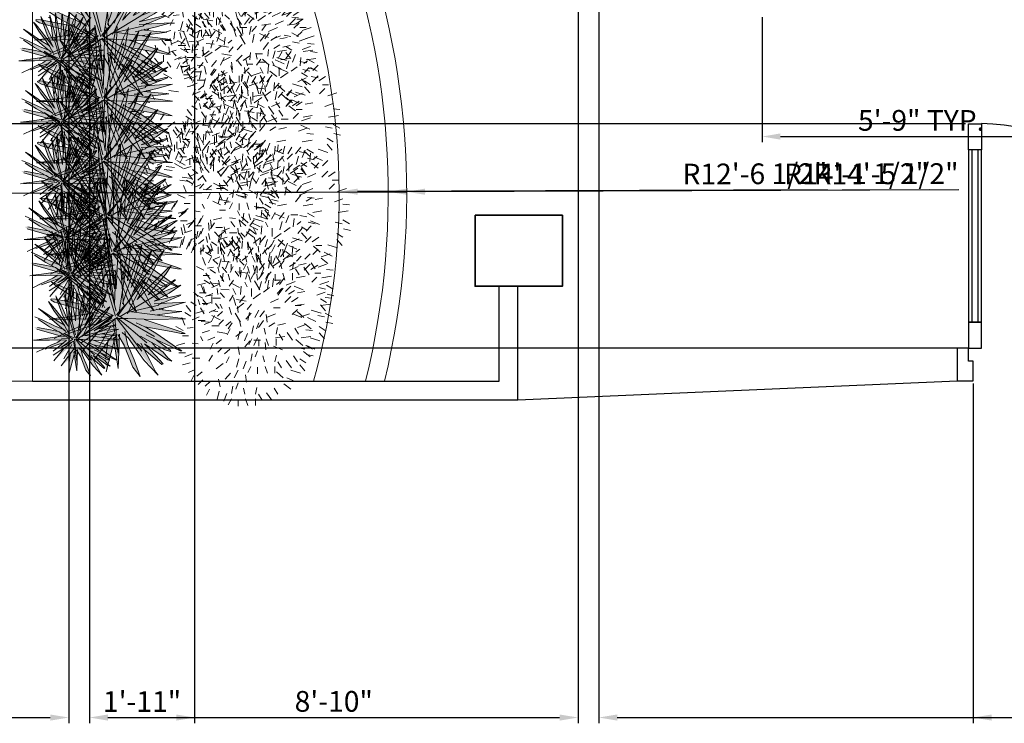
# Model space of a CAD drawing. Units: inches. Extents: x 1239 to 2276906, y 2273 to 321338.
# Tile 6 of 23: x 1541 to 1754, y 2276 to 2428. Entities that reach past the tile are written whole.
import ezdxf

# ---------------------------------------------------------------- set-up
doc = ezdxf.new("R2010")
doc.units = ezdxf.units.IN
for name, color, linetype, lineweight in [('A-ANNO-DIMS', 2, 'Continuous', 18), ('A-COLS', 7, 'Continuous', 35), ('C-PROP', 7, 'Continuous', 25), ('L-PLNT', 94, 'Continuous', 13), ('L-SITE-GATE', 1, 'Continuous', 25)]:
    doc.layers.add(name, color=color, linetype=linetype, lineweight=lineweight)
doc.styles.get("Standard").update_dxf_attribs({"font": 'arial.ttf'})
doc.dimstyles.new('ISO-25', dxfattribs={"dimtxt": 4.5, "dimasz": 4, "dimexe": 1.25, "dimexo": 0.625, "dimtad": 1, "dimdec": 1, "dimlunit": 3, "dimtxsty": 'Standard', "dimcen": 2.5, "dimadec": 0, "dimazin": 0, "dimtfac": 1, "dimtdec": 1, "dimtmove": 0, "dimatfit": 3, "dimfxl": 1, "dimarcsym": 0})

# ---------------------------------------------------------------- blocks, each defined once
blk = doc.blocks.new('A$C545C060E')
h = blk.add_hatch(color=256)
h.set_gradient(color1=(31, 127, 0), color2=(45, 179, 0), one_color=1, tint=0.35, name='INVSPHERICAL')
h.paths.add_polyline_path([(0.529, 2.393), (0.645, 2.304), (1.889, 1.967), (0.489, 1.77), (1.843, 1.787), (1.618, 1.643), (0.635, 1.178), (1.063, 1.326), (1.966, 1.643), (1.461, 1.231), (1.869, 1.417), (2.379, 1.664), (2.177, 1.5), (1.446, 1.03), (1.981, 1.358), (1.481, 0.744), (2.376, 1.553), (1.986, 0.848), (2.48, 1.336), (1.85, 0.496), (2.266, 0.842), (2.223, 0.533), (2.243, 0.142), (2.487, 1.093), (2.615, 0.257), (2.655, 1.214), (3.074, 0.284), (3.303, 0), (2.908, 1.003), (2.846, 1.271), (2.929, 1.199), (3.853, 0.038), (3.428, 0.832), (3.973, 0.376), (4.009, 0.393), (3.432, 1.008), (3.923, 0.676), (4.175, 0.507), (4.274, 0.474), (4.155, 0.583), (4.009, 0.757), (3.765, 0.932), (3.662, 1.051), (4.067, 0.828), (4.243, 0.779), (4.238, 0.801), (3.802, 1.133), (4.534, 0.795), (4.591, 0.795), (4.42, 0.899), (4.103, 1.12), (3.786, 1.34), (3.464, 1.533), (3.968, 1.441), (4.415, 1.362), (4.571, 1.335), (4.695, 1.33), (3.997, 1.572), (3.423, 1.771), (4.695, 1.782), (3.833, 1.912), (4.591, 2.011), (3.836, 2.079), (4.706, 2.305), (3.951, 2.263), (4.55, 2.506), (4.555, 2.528), (4.493, 2.517), (3.734, 2.332), (4.197, 2.577), (4.56, 2.833), (3.786, 2.523), (4.363, 2.959), (4.394, 2.997), (4.363, 2.997), (3.558, 2.528), (3.549, 2.536), (4.087, 3.155), (4.254, 3.422), (4.191, 3.389), (3.209, 2.381), (4.046, 3.912), (3.999, 3.874), (3.09, 2.626), (3.547, 3.58), (3.666, 3.934), (3.35, 3.438), (3.017, 2.752), (3.225, 3.411), (3.345, 4.064), (3.243, 3.868), (3.184, 3.754), (2.919, 3.073), (2.986, 3.83), (2.991, 4.097), (2.96, 4.075), (2.742, 2.981), (2.732, 2.92), (2.659, 4.026), (2.633, 4.092), (2.612, 4.005), (2.56, 2.719), (2.3, 4.135), (2.382, 2.743), (2.025, 4.026), (2.02, 3.934), (1.968, 3.917), (2.046, 3.874), (2.185, 2.776), (1.976, 3.197), (1.829, 3.524), (1.673, 3.773), (1.577, 3.963), (1.613, 3.821), (1.751, 3.44), (1.89, 3.059), (2.192, 2.446), (1.345, 3.551), (1.215, 3.683), (1.481, 3.234), (2.006, 2.515), (1.567, 2.769), (0.983, 3.176), (0.731, 3.334), (1.255, 2.901), (1.969, 2.294), (0.912, 2.769), (0.549, 2.927), (1.687, 2.199), (0.675, 2.399), (0.554, 2.409)])
h = blk.add_hatch(color=256)
h.set_gradient(color1=(31, 127, 0), color2=(55, 219, 0), one_color=1, tint=0.43, name='SPHERICAL')
h.paths.add_polyline_path([(3.023, 2.188), (3.114, 2.362), (3.471, 3.049), (3.33, 2.866), (2.618, 1.891), (2.679, 1.855), (2.94, 2.013)])
h = blk.add_hatch(color=256)
h.set_gradient(color1=(31, 127, 0), color2=(45, 179, 0), one_color=1, tint=0.35, name='INVSPHERICAL')
h.paths.add_polyline_path([(0.025, 1.517), (0.098, 1.461), (0.877, 1.25), (0, 1.126), (0.848, 1.137), (0.707, 1.047), (0.092, 0.756), (0.36, 0.848), (0.925, 1.047), (0.609, 0.789), (0.865, 0.905), (1.184, 1.06), (1.058, 0.958), (0.6, 0.663), (0.935, 0.868), (0.622, 0.484), (1.182, 0.99), (0.938, 0.549), (1.247, 0.855), (0.853, 0.328), (1.113, 0.545), (1.086, 0.352), (1.099, 0.106), (1.252, 0.703), (1.332, 0.179), (1.357, 0.779), (1.62, 0.195), (1.763, 0.018), (1.515, 0.646), (1.477, 0.814), (1.529, 0.769), (2.108, 0.042), (1.841, 0.539), (2.183, 0.253), (2.206, 0.264), (1.844, 0.649), (2.152, 0.441), (2.31, 0.335), (2.371, 0.315), (2.297, 0.383), (2.206, 0.492), (2.053, 0.602), (1.988, 0.676), (2.242, 0.537), (2.352, 0.506), (2.349, 0.52), (2.076, 0.728), (2.534, 0.516), (2.57, 0.516), (2.463, 0.581), (2.264, 0.719), (2.066, 0.857), (1.864, 0.978), (2.18, 0.921), (2.46, 0.871), (2.557, 0.854), (2.636, 0.851), (2.198, 1.003), (1.839, 1.127), (2.636, 1.134), (2.095, 1.216), (2.57, 1.277), (2.097, 1.32), (2.642, 1.462), (2.169, 1.435), (2.544, 1.588), (2.548, 1.602), (2.509, 1.595), (2.033, 1.479), (2.323, 1.632), (2.551, 1.793), (2.066, 1.598), (2.427, 1.871), (2.447, 1.895), (2.427, 1.895), (1.923, 1.602), (1.917, 1.606), (2.255, 1.994), (2.359, 2.161), (2.32, 2.141), (1.704, 1.509), (2.229, 2.469), (2.199, 2.445), (1.63, 1.663), (1.916, 2.26), (1.991, 2.482), (1.792, 2.172), (1.584, 1.741), (1.714, 2.155), (1.789, 2.564), (1.726, 2.441), (1.688, 2.369), (1.522, 1.943), (1.565, 2.417), (1.568, 2.584), (1.548, 2.571), (1.412, 1.885), (1.405, 1.847), (1.36, 2.54), (1.343, 2.581), (1.33, 2.526), (1.298, 1.721), (1.135, 2.608), (1.186, 1.736), (0.962, 2.54), (0.959, 2.482), (0.927, 2.472), (0.976, 2.445), (1.063, 1.757), (0.932, 2.02), (0.84, 2.226), (0.742, 2.381), (0.682, 2.501), (0.704, 2.411), (0.791, 2.173), (0.878, 1.934), (1.067, 1.55), (0.537, 2.242), (0.455, 2.325), (0.622, 2.044), (0.951, 1.593), (0.676, 1.752), (0.31, 2.007), (0.152, 2.107), (0.48, 1.835), (0.927, 1.455), (0.265, 1.752), (0.038, 1.851), (0.751, 1.395), (0.117, 1.52), (0.041, 1.527)])
h = blk.add_hatch(color=256)
h.set_gradient(color1=(31, 127, 0), color2=(55, 219, 0), one_color=1, tint=0.43, name='SPHERICAL')
h.paths.add_polyline_path([(1.334, 1.202), (1.372, 1.18), (1.536, 1.279), (1.588, 1.388), (1.645, 1.497), (1.868, 1.928), (1.78, 1.813)])
for p, q in [((2.02, 3.934, -52.769), (2.025, 4.026, -52.769)), ((2.025, 4.026, -52.769), (2.389, 2.719, -52.769)), ((2.295, 4.037, -52.769), (2.3, 4.135, -52.769)), ((2.389, 2.643, -52.769), (2.295, 4.037, -52.769)), ((2.3, 4.135, -52.769), (2.534, 2.893, -52.769)), ((2.591, 3.329, -52.769), (2.612, 4.005, -52.769)), ((2.612, 4.005, -52.769), (2.633, 4.092, -52.769)), ((2.633, 4.092, -52.769), (2.659, 4.026, -52.769)), ((2.659, 4.026, -52.769), (2.732, 2.92, -52.769)), ((2.742, 2.981, -52.769), (2.945, 4.01, -52.769)), ((2.945, 4.01, -52.769), (2.96, 4.075, -52.769)), ((2.96, 4.075, -52.769), (2.991, 4.097, -52.769)), ((2.991, 4.097, -52.769), (2.986, 3.83, -52.769)), ((3.184, 3.754, -52.769), (3.303, 3.983, -52.769)), ((3.345, 4.064, -52.769), (3.225, 3.411, -52.769)), ((3.303, 3.983, -52.769), (3.345, 4.064, -52.769)), ((1.215, 3.683, -52.769), (1.481, 3.234, -52.769)), ((1.345, 3.551, -52.769), (1.215, 3.683, -52.769)), ((1.577, 3.963, -52.769), (1.613, 3.821, -52.769)), ((1.673, 3.773, -52.769), (1.577, 3.963, -52.769)), ((1.613, 3.821, -52.769), (1.89, 3.059, -52.769)), ((1.829, 3.524, -52.769), (1.673, 3.773, -52.769)), ((1.968, 3.917, -52.769), (2.02, 3.934, -52.769)), ((2.046, 3.874, -52.769), (1.968, 3.917, -52.769)), ((2.103, 3.378, -52.769), (2.046, 3.874, -52.769)), ((2.986, 3.83, -52.769), (2.908, 2.964, -52.769)), ((3.095, 3.498, -52.769), (3.184, 3.754, -52.769)), ((3.428, 3.553, -52.769), (3.666, 3.934, -52.769)), ((3.508, 3.479, -52.769), (3.625, 3.884, -52.769)), ((3.666, 3.934, -52.769), (3.547, 3.58, -52.769)), ((3.558, 3.269, -52.769), (3.999, 3.874, -52.769)), ((4.046, 3.912, -52.769), (3.635, 3.155, -52.769)), ((3.999, 3.874, -52.769), (4.046, 3.912, -52.769)), ((1.602, 3.229, -52.769), (1.345, 3.551, -52.769)), ((1.976, 3.197, -52.769), (1.829, 3.524, -52.769)), ((2.186, 2.773, -52.769), (2.103, 3.378, -52.769)), ((3.198, 3.588, -52.769), (2.75, 2.248, -52.769)), ((2.919, 3.073, -52.769), (3.095, 3.498, -52.769)), ((3.225, 3.411, -52.769), (3.017, 2.752, -52.769)), ((3.547, 3.58, -52.769), (3.085, 2.626, -52.769)), ((3.298, 3.329, -52.769), (3.35, 3.438, -52.769)), ((3.35, 3.438, -52.769), (3.428, 3.553, -52.769)), ((3.771, 2.975, -52.769), (4.191, 3.389, -52.769)), ((4.254, 3.422, -52.769), (4.087, 3.155, -52.769)), ((4.191, 3.389, -52.769), (4.254, 3.422, -52.769)), ((0.731, 3.334, -52.769), (1.255, 2.901, -52.769)), ((0.983, 3.176, -52.769), (0.731, 3.334, -52.769)), ((1.567, 2.769, -52.769), (0.983, 3.176, -52.769)), ((1.481, 3.234, -52.769), (1.819, 2.785, -52.769)), ((2.157, 2.505, -52.769), (1.602, 3.229, -52.769)), ((1.89, 3.059, -52.769), (2.192, 2.446, -52.769)), ((2.102, 2.927, -52.769), (1.976, 3.197, -52.769)), ((2.56, 2.719, -52.769), (2.591, 3.329, -52.769)), ((2.849, 3.284, -52.769), (2.65, 1.996, -52.769)), ((3.017, 2.752, -52.769), (3.298, 3.329, -52.769)), ((3.09, 2.626, -52.769), (3.558, 3.269, -52.769)), ((3.635, 3.155, -52.769), (3.209, 2.381, -52.769)), ((4.087, 3.155, -52.769), (3.542, 2.528, -52.769)), ((0.549, 2.927, -52.769), (0.72, 2.785, -52.769)), ((0.912, 2.769, -52.769), (0.549, 2.927, -52.769)), ((0.72, 2.785, -52.769), (1.27, 2.43, -52.769)), ((1.522, 2.483, -52.769), (0.912, 2.769, -52.769)), ((1.255, 2.901, -52.769), (1.653, 2.552, -52.769)), ((2.006, 2.515, -52.769), (1.567, 2.769, -52.769)), ((1.819, 2.785, -52.769), (2.016, 2.494, -52.769)), ((2.192, 2.764, -52.769), (2.102, 2.927, -52.769)), ((2.269, 2.899, -52.769), (2.394, 2.654, -52.769)), ((2.279, 2.724, -52.769), (2.269, 2.899, -52.769)), ((2.534, 2.893, -52.769), (2.56, 2.719, -52.769)), ((2.6, 1.866, -52.769), (3.33, 2.866, -52.769)), ((2.732, 2.92, -52.769), (2.783, 2.212, -52.769)), ((3.471, 3.049, -52.769), (3.114, 2.362, -52.769)), ((3.209, 2.381, -52.769), (3.771, 2.975, -52.769)), ((3.33, 2.866, -52.769), (3.471, 3.049, -52.769)), ((3.558, 2.528, -52.769), (4.327, 2.975, -52.769)), ((4.363, 2.959, -52.769), (3.786, 2.523, -52.769)), ((4.191, 2.692, -52.769), (4.514, 2.822, -52.769)), ((4.56, 2.833, -52.769), (4.197, 2.577, -52.769)), ((4.327, 2.975, -52.769), (4.363, 2.997, -52.769)), ((4.394, 2.997, -52.769), (4.363, 2.959, -52.769)), ((4.363, 2.997, -52.769), (4.394, 2.997, -52.769)), ((4.514, 2.822, -52.769), (4.56, 2.833, -52.769)), ((0.682, 2.501), (0.704, 2.411)), ((0.742, 2.381), (0.682, 2.501)), ((0.927, 2.472), (0.959, 2.482)), ((0.976, 2.445), (0.927, 2.472)), ((0.959, 2.482), (0.962, 2.54)), ((0.962, 2.54), (1.19, 1.721)), ((1.011, 2.134), (0.976, 2.445)), ((1.132, 2.547), (1.135, 2.608)), ((1.19, 1.673), (1.132, 2.547)), ((1.135, 2.608), (1.281, 1.83)), ((1.317, 2.103), (1.33, 2.526)), ((1.33, 2.526), (1.343, 2.581)), ((1.343, 2.581), (1.36, 2.54)), ((1.36, 2.54), (1.405, 1.847)), ((1.412, 1.885), (1.539, 2.53)), ((2.046, 2.261, -52.769), (1.522, 2.483, -52.769)), ((1.539, 2.53), (1.548, 2.571)), ((1.548, 2.571), (1.568, 2.584)), ((1.568, 2.584), (1.565, 2.417)), ((1.653, 2.552, -52.769), (2.087, 2.198, -52.769)), ((1.688, 2.369), (1.763, 2.513)), ((1.789, 2.564), (1.714, 2.155)), ((1.763, 2.513), (1.789, 2.564)), ((1.841, 2.243), (1.991, 2.482)), ((1.891, 2.197), (1.965, 2.451)), ((1.991, 2.482), (1.916, 2.26)), ((1.923, 2.066), (2.199, 2.445)), ((2.229, 2.469), (1.971, 1.994)), ((2.016, 2.494, -52.769), (2.208, 2.129, -52.769)), ((2.199, 2.445), (2.229, 2.469)), ((2.539, 1.864, -52.769), (2.279, 2.724, -52.769)), ((2.394, 2.654, -52.769), (2.55, 2.027, -52.769)), ((3.786, 2.523, -52.769), (2.674, 1.853, -52.769)), ((3.085, 2.626, -52.769), (2.955, 2.288, -52.769)), ((3.734, 2.332, -52.769), (4.493, 2.517, -52.769)), ((3.797, 2.528, -52.769), (4.191, 2.692, -52.769)), ((4.197, 2.577, -52.769), (3.848, 2.381, -52.769)), ((4.55, 2.506, -52.769), (3.854, 2.223, -52.769)), ((4.493, 2.517, -52.769), (4.555, 2.528, -52.769)), ((4.555, 2.528, -52.769), (4.55, 2.506, -52.769)), ((0.455, 2.325), (0.622, 2.044)), ((0.537, 2.242), (0.455, 2.325)), ((0.554, 2.409, -52.769), (0.529, 2.393, -52.769)), ((0.529, 2.393, -52.769), (0.539, 2.367, -52.769)), ((0.698, 2.04), (0.537, 2.242)), ((0.539, 2.367, -52.769), (0.645, 2.304, -52.769)), ((0.675, 2.399, -52.769), (0.554, 2.409, -52.769)), ((0.645, 2.304, -52.769), (1.734, 1.992, -52.769)), ((1.32, 2.272, -52.769), (0.675, 2.399, -52.769)), ((0.704, 2.411), (0.878, 1.934)), ((0.84, 2.226), (0.742, 2.381)), ((0.932, 2.02), (0.84, 2.226)), ((1.27, 2.43, -52.769), (1.764, 2.156, -52.769)), ((1.769, 2.182, -52.769), (1.32, 2.272, -52.769)), ((1.697, 2.266), (1.416, 1.426)), ((1.565, 2.417), (1.516, 1.875)), ((1.522, 1.943), (1.633, 2.209)), ((1.714, 2.155), (1.584, 1.741)), ((1.916, 2.26), (1.627, 1.663)), ((1.633, 2.209), (1.688, 2.369)), ((1.76, 2.103), (1.792, 2.172)), ((1.764, 2.156, -52.769), (2.182, 1.902, -52.769)), ((1.792, 2.172), (1.841, 2.243)), ((2.056, 1.881), (2.32, 2.141)), ((2.359, 2.161), (2.255, 1.994)), ((2.32, 2.141), (2.359, 2.161)), ((2.565, 1.907, -52.769), (2.84, 2.229, -52.769)), ((2.84, 2.229, -52.769), (2.606, 1.885, -52.769)), ((3.878, 2.205, -52.769), (2.857, 1.97, -52.769)), ((3.023, 2.188, -52.769), (2.907, 1.944, -52.769)), ((3.114, 2.362, -52.769), (3.023, 2.188, -52.769)), ((4.228, 2.169, -52.769), (3.61, 2.027, -52.769)), ((3.848, 2.381, -52.769), (3.734, 2.332, -52.769)), ((3.734, 2.25, -52.769), (4.301, 2.283, -52.769)), ((3.949, 2.282, -52.769), (4.001, 2.285, -52.769)), ((4.001, 2.285, -52.769), (4.042, 2.282, -52.769)), ((4.706, 2.305, -52.769), (4.228, 2.169, -52.769)), ((4.301, 2.283, -52.769), (4.706, 2.305, -52.769)), ((0.265, 1.752), (0.038, 1.851)), ((0.152, 2.107), (0.48, 1.835)), ((0.31, 2.007), (0.152, 2.107)), ((0.676, 1.752), (0.31, 2.007)), ((0.48, 1.835), (0.729, 1.617)), ((0.622, 2.044), (0.834, 1.762)), ((1.068, 1.844, -52.769), (0.64, 1.791, -52.769)), ((1.045, 1.587), (0.698, 2.04)), ((0.878, 1.934), (1.067, 1.55)), ((1.011, 1.851), (0.932, 2.02)), ((1.063, 1.755), (1.011, 2.134)), ((1.067, 1.749), (1.011, 1.851)), ((1.981, 1.981, -52.769), (1.068, 1.844, -52.769)), ((1.115, 1.834), (1.194, 1.68)), ((1.122, 1.724), (1.115, 1.834)), ((1.281, 1.83), (1.298, 1.721)), ((1.298, 1.721), (1.317, 2.103)), ((1.479, 2.075), (1.354, 1.268)), ((1.405, 1.847), (1.438, 1.404)), ((1.584, 1.741), (1.76, 2.103)), ((1.63, 1.663), (1.923, 2.066)), ((1.868, 1.928), (1.645, 1.497)), ((1.971, 1.994), (1.704, 1.509)), ((1.704, 1.509), (2.056, 1.881)), ((1.734, 1.992, -52.769), (2.006, 1.949, -52.769)), ((1.78, 1.813), (1.868, 1.928)), ((1.87, 1.874, -52.769), (2.276, 1.84, -52.769)), ((2.255, 1.994), (1.913, 1.602)), ((1.923, 1.602), (2.404, 1.881)), ((2.009, 2.092, -52.769), (2.476, 1.885, -52.769)), ((2.425, 1.814, -52.769), (2.009, 2.092, -52.769)), ((2.427, 1.871), (2.066, 1.598)), ((2.404, 1.881), (2.427, 1.895)), ((2.447, 1.895), (2.427, 1.871)), ((2.427, 1.895), (2.447, 1.895)), ((3.504, 1.039, -52.769), (2.584, 1.831, -52.769)), ((3.737, 1.239, -52.769), (2.617, 1.892, -52.769)), ((3.516, 1.945, -52.769), (3.028, 2.005, -52.769)), ((4.701, 1.782, -52.769), (3.516, 1.945, -52.769)), ((3.807, 2.082, -52.769), (4.264, 2.038, -52.769)), ((4.591, 2.011, -52.769), (3.833, 1.912, -52.769)), ((3.886, 2.102, -52.769), (3.98, 2.099, -52.769)), ((3.98, 2.099, -52.769), (4.025, 2.091, -52.769)), ((4.264, 2.038, -52.769), (4.534, 2.016, -52.769)), ((4.534, 2.016, -52.769), (4.591, 2.011, -52.769)), ((0.145, 1.762), (0.49, 1.54)), ((0.647, 1.573), (0.265, 1.752)), ((0.64, 1.791, -52.769), (0.489, 1.77, -52.769)), ((0.489, 1.77, -52.769), (1.275, 1.775, -52.769)), ((0.49, 1.54), (0.799, 1.368)), ((0.976, 1.434), (0.647, 1.573)), ((0.951, 1.593), (0.676, 1.752)), ((0.729, 1.617), (1.001, 1.395)), ((0.834, 1.762), (0.957, 1.58)), ((0.957, 1.58), (1.077, 1.352)), ((1.285, 1.185), (1.122, 1.724)), ((1.194, 1.68), (1.291, 1.288)), ((1.275, 1.775, -52.769), (2.051, 1.791, -52.769)), ((1.323, 1.186), (1.78, 1.813)), ((1.618, 1.643, -52.769), (1.345, 1.521, -52.769)), ((2.066, 1.598), (1.369, 1.178)), ((1.966, 1.643, -52.769), (1.461, 1.231, -52.769)), ((1.627, 1.663), (1.545, 1.451)), ((1.608, 1.516, -52.769), (1.966, 1.643, -52.769)), ((1.678, 1.675, -52.769), (1.618, 1.643, -52.769)), ((1.865, 1.801, -52.769), (1.678, 1.675, -52.769)), ((1.869, 1.417, -52.769), (2.425, 1.814, -52.769)), ((2.456, 1.716, -52.769), (1.869, 1.417, -52.769)), ((1.966, 1.643, -52.769), (2.107, 1.77, -52.769)), ((1.986, 0.848, -52.769), (2.376, 1.553, -52.769)), ((2.033, 1.479), (2.509, 1.595)), ((2.072, 1.602), (2.32, 1.704)), ((2.323, 1.632), (2.105, 1.509)), ((2.544, 1.588), (2.108, 1.41)), ((2.177, 1.5, -52.769), (2.379, 1.664, -52.769)), ((2.32, 1.704), (2.522, 1.786)), ((2.551, 1.793), (2.323, 1.632)), ((2.617, 0.725, -52.769), (2.456, 1.716, -52.769)), ((2.509, 1.595), (2.548, 1.602)), ((2.513, 1.809, -52.769), (2.617, 0.725, -52.769)), ((2.522, 1.786), (2.551, 1.793)), ((2.548, 1.602), (2.544, 1.588)), ((2.913, 1.793, -52.769), (2.555, 1.798, -52.769)), ((3.347, 0.787, -52.769), (2.559, 1.822, -52.769)), ((3.672, 1.76, -52.769), (2.913, 1.793, -52.769)), ((3.443, 1.537, -52.769), (3.178, 1.657, -52.769)), ((3.422, 1.766, -52.769), (4.571, 1.379, -52.769)), ((3.677, 1.493, -52.769), (3.443, 1.537, -52.769)), ((3.448, 1.542, -52.769), (3.786, 1.34, -52.769)), ((4.695, 1.782, -52.769), (3.672, 1.76, -52.769)), ((0.098, 1.461), (0.78, 1.265)), ((0.521, 1.441), (0.117, 1.52)), ((0.935, 1.259), (0.363, 1.173)), ((0.802, 1.385), (0.521, 1.441)), ((1.048, 1.379, -52.769), (0.635, 1.178, -52.769)), ((0.78, 1.265), (0.951, 1.239)), ((0.799, 1.368), (1.061, 1.209)), ((0.952, 1.328), (1.245, 1.199)), ((1.213, 1.154), (0.952, 1.328)), ((1.345, 1.521, -52.769), (1.048, 1.379, -52.769)), ((1.063, 1.326, -52.769), (1.608, 1.516, -52.769)), ((1.301, 1.212), (1.473, 1.414)), ((1.473, 1.414), (1.327, 1.199)), ((1.446, 1.03, -52.769), (2.177, 1.5, -52.769)), ((1.981, 1.358, -52.769), (1.481, 0.744, -52.769)), ((2.123, 1.399), (1.484, 1.252)), ((1.588, 1.388), (1.515, 1.235)), ((1.645, 1.497), (1.588, 1.388)), ((1.897, 1.236), (1.591, 1.274)), ((2.639, 1.134), (1.897, 1.236)), ((2.343, 1.376), (1.955, 1.288)), ((2.105, 1.509), (2.033, 1.479)), ((2.033, 1.427), (2.388, 1.448)), ((2.079, 1.322), (2.365, 1.294)), ((2.57, 1.277), (2.095, 1.216)), ((2.128, 1.335), (2.187, 1.333)), ((2.168, 1.447), (2.2, 1.449)), ((2.187, 1.333), (2.215, 1.328)), ((2.2, 1.449), (2.226, 1.447)), ((2.313, 1.109, -52.769), (2.48, 1.336, -52.769)), ((2.642, 1.462), (2.343, 1.376)), ((2.365, 1.294), (2.534, 1.281)), ((2.388, 1.448), (2.642, 1.462)), ((2.485, 1.067, -52.769), (2.5, 1.22, -52.769)), ((2.534, 1.281), (2.57, 1.277)), ((2.799, 0.97, -52.769), (2.606, 1.297, -52.769)), ((2.658, 1.308, -52.769), (2.617, 0.245, -52.769)), ((2.929, 1.199, -52.769), (2.742, 1.362, -52.769)), ((2.819, 1.39, -52.769), (2.908, 1.003, -52.769)), ((3.62, 1.074, -52.769), (3.313, 1.248, -52.769)), ((3.802, 1.133, -52.769), (3.479, 1.292, -52.769)), ((4.259, 1.39, -52.769), (3.677, 1.493, -52.769)), ((3.786, 1.34, -52.769), (4.42, 0.899, -52.769)), ((4.571, 1.335, -52.769), (4.259, 1.39, -52.769)), ((4.571, 1.379, -52.769), (4.695, 1.33, -52.769)), ((4.695, 1.33, -52.769), (4.571, 1.335, -52.769)), ((0, 1.126), (0.493, 1.13)), ((0.363, 1.173), (0.095, 1.14)), ((0.537, 0.971), (0.351, 0.881)), ((0.36, 0.848), (0.701, 0.967)), ((0.493, 1.13), (0.979, 1.14)), ((0.707, 1.047), (0.537, 0.971)), ((0.6, 0.663), (1.058, 0.958)), ((0.925, 1.047), (0.609, 0.789)), ((0.701, 0.967), (0.925, 1.047)), ((0.745, 1.067), (0.707, 1.047)), ((0.862, 1.146), (0.745, 1.067)), ((0.865, 0.905), (1.213, 1.154)), ((1.232, 1.093), (0.865, 0.905)), ((0.866, 1.192), (1.12, 1.17)), ((0.925, 1.047), (1.014, 1.126)), ((0.938, 0.549), (1.182, 0.99)), ((1.058, 0.958), (1.184, 1.06)), ((1.333, 0.472), (1.232, 1.093)), ((1.268, 1.151), (1.333, 0.472)), ((1.519, 1.141), (1.294, 1.144)), ((1.791, 0.511), (1.297, 1.159)), ((1.889, 0.669), (1.312, 1.165)), ((2.035, 0.794), (1.333, 1.203)), ((1.994, 1.12), (1.519, 1.141)), ((1.851, 0.98), (1.685, 1.056)), ((1.838, 1.124), (2.557, 0.881)), ((1.85, 0.496, -52.769), (2.313, 1.109, -52.769)), ((1.997, 0.953), (1.851, 0.98)), ((1.854, 0.984), (2.066, 0.857)), ((2.636, 1.134), (1.994, 1.12)), ((2.362, 0.888), (1.997, 0.953)), ((2.308, 1.151, -52.769), (2.223, 0.533, -52.769)), ((2.243, 0.142, -52.769), (2.485, 1.067, -52.769)), ((2.617, 0.245, -52.769), (2.471, 1.199, -52.769)), ((3.074, 0.284, -52.769), (2.799, 0.97, -52.769)), ((2.908, 1.003, -52.769), (3.111, 0.512, -52.769)), ((3.427, 0.496, -52.769), (2.929, 1.199, -52.769)), ((3.973, 0.376, -52.769), (3.204, 1.019, -52.769)), ((3.324, 1.03, -52.769), (3.599, 0.507, -52.769)), ((3.687, 0.839, -52.769), (3.432, 1.008, -52.769)), ((3.432, 1.008, -52.769), (3.786, 0.643, -52.769)), ((4.067, 0.828, -52.769), (3.62, 1.074, -52.769)), ((3.656, 1.057, -52.769), (3.765, 0.932, -52.769)), ((3.765, 0.932, -52.769), (4.009, 0.757, -52.769)), ((4.243, 0.932, -52.769), (3.802, 1.133, -52.769)), ((3.802, 1.128, -52.769), (4.176, 0.856, -52.769)), ((4.534, 0.795, -52.769), (4.243, 0.932, -52.769)), ((0.351, 0.881), (0.092, 0.756)), ((0.935, 0.868), (0.622, 0.484)), ((0.853, 0.328), (1.143, 0.713)), ((1.14, 0.739), (1.086, 0.352)), ((1.099, 0.106), (1.251, 0.686)), ((1.143, 0.713), (1.247, 0.855)), ((1.333, 0.171), (1.242, 0.769)), ((1.251, 0.686), (1.26, 0.782)), ((1.447, 0.625), (1.327, 0.83)), ((1.359, 0.837), (1.333, 0.171)), ((1.529, 0.769), (1.411, 0.871)), ((1.62, 0.195), (1.447, 0.625)), ((1.46, 0.888), (1.515, 0.646)), ((1.515, 0.646), (1.643, 0.339)), ((1.841, 0.328), (1.529, 0.769)), ((2.183, 0.253), (1.701, 0.656)), ((1.962, 0.69), (1.77, 0.799)), ((1.776, 0.663), (1.948, 0.335)), ((2.004, 0.543), (1.844, 0.649)), ((1.844, 0.649), (2.066, 0.421)), ((2.076, 0.728), (1.874, 0.827)), ((2.242, 0.537), (1.962, 0.69)), ((1.984, 0.68), (2.053, 0.602)), ((2.066, 0.857), (2.463, 0.581)), ((2.352, 0.602), (2.076, 0.728)), ((2.076, 0.724), (2.31, 0.554)), ((2.557, 0.854), (2.362, 0.888)), ((2.557, 0.881), (2.636, 0.851)), ((2.636, 0.851), (2.557, 0.854)), ((4.16, 0.512, -52.769), (3.687, 0.839, -52.769)), ((3.786, 0.643, -52.769), (4.009, 0.393, -52.769)), ((4.009, 0.757, -52.769), (4.155, 0.583, -52.769)), ((4.243, 0.779, -52.769), (4.067, 0.828, -52.769)), ((4.176, 0.856, -52.769), (4.238, 0.801, -52.769)), ((4.238, 0.801, -52.769), (4.243, 0.779, -52.769)), ((4.42, 0.899, -52.769), (4.591, 0.795, -52.769)), ((4.591, 0.795, -52.769), (4.534, 0.795, -52.769)), ((1.643, 0.339), (1.763, 0.018)), ((2.108, 0.042), (1.841, 0.328)), ((1.948, 0.335), (2.066, 0.1)), ((2.3, 0.339), (2.004, 0.543)), ((2.053, 0.602), (2.206, 0.492)), ((2.066, 0.421), (2.206, 0.264)), ((2.206, 0.492), (2.297, 0.383)), ((2.352, 0.506), (2.242, 0.537)), ((2.297, 0.383), (2.371, 0.315)), ((2.371, 0.315), (2.3, 0.339)), ((2.31, 0.554), (2.349, 0.52)), ((2.349, 0.52), (2.352, 0.506)), ((2.534, 0.516), (2.352, 0.602)), ((2.463, 0.581), (2.57, 0.516)), ((2.57, 0.516), (2.534, 0.516)), ((3.111, 0.512, -52.769), (3.303, 0, -52.769)), ((3.853, 0.038, -52.769), (3.427, 0.496, -52.769)), ((3.599, 0.507, -52.769), (3.786, 0.131, -52.769)), ((4.009, 0.393, -52.769), (3.973, 0.376, -52.769)), ((4.155, 0.583, -52.769), (4.274, 0.474, -52.769)), ((4.274, 0.474, -52.769), (4.16, 0.512, -52.769)), ((1.763, 0.018), (1.62, 0.195)), ((2.066, 0.1), (2.108, 0.042)), ((2.206, 0.264), (2.183, 0.253)), ((3.303, 0, -52.769), (3.074, 0.284, -52.769)), ((3.786, 0.131, -52.769), (3.853, 0.038, -52.769))]:
    blk.add_line(p, q)
blk = doc.blocks.new('t1')
at = {"xscale": 1200, "yscale": 1200, "zscale": 1200}
blk.add_blockref('A$C545C060E', (1649217, 160231), dxfattribs=at)
blk = doc.blocks.new('A$C20C17E7E')
for p, q in [((1.899, 5.117), (1.929, 5.423)), ((2.205, 5.147), (2.144, 5.393)), ((2.635, 5.271), (2.665, 5.546)), ((2.849, 5.179), (2.941, 5.485)), ((3.063, 5.179), (3.217, 5.455)), ((3.37, 5.179), (3.584, 5.455)), ((3.646, 5.025), (3.768, 5.332)), ((1.195, 4.597), (1.134, 4.871)), ((1.562, 4.871), (1.409, 5.086)), ((1.807, 4.871), (1.746, 5.147)), ((2.174, 4.903), (2.359, 5.147)), ((2.635, 4.565), (2.665, 4.903)), ((2.91, 4.871), (2.819, 5.056)), ((3.401, 4.749), (3.492, 5.086)), ((3.584, 4.658), (3.829, 4.841)), ((3.952, 4.871), (3.983, 5.21)), ((4.105, 4.964), (4.259, 5.086)), ((4.472, 4.688), (4.687, 4.903)), ((0.919, 4.474), (0.735, 4.658)), ((1.47, 4.198), (1.47, 4.474)), ((1.716, 4.565), (1.685, 4.81)), ((1.991, 4.443), (1.807, 4.627)), ((2.45, 4.565), (2.328, 4.81)), ((2.45, 4.106), (2.359, 4.443)), ((2.604, 4.228), (2.819, 4.504)), ((3.095, 4.474), (3.095, 4.81)), ((3.156, 4.382), (3.462, 4.597)), ((4.135, 4.597), (4.32, 4.81)), ((4.442, 4.228), (4.687, 4.474)), ((4.717, 4.259), (4.993, 4.443)), ((0.613, 3.861), (0.428, 4.106)), ((0.827, 4.106), (0.613, 4.259)), ((0.98, 4.137), (0.919, 4.352)), ((1.286, 4.137), (1.102, 4.352)), ((1.777, 3.983), (1.623, 4.198)), ((2.267, 3.739), (2.174, 4.045)), ((2.543, 3.831), (2.513, 4.076)), ((2.91, 3.953), (3.095, 4.167)), ((3.86, 4.228), (4.196, 4.382)), ((4.871, 4.106), (5.117, 4.106)), ((0.367, 3.31), (0.244, 3.616)), ((0.613, 3.677), (0.367, 3.831)), ((0.949, 3.646), (0.674, 3.524)), ((1.164, 3.77), (1.01, 4.014)), ((1.807, 3.524), (1.47, 3.707)), ((2.635, 3.431), (2.42, 3.8)), ((2.941, 3.494), (3.002, 3.831)), ((3.431, 3.646), (3.614, 3.892)), ((3.707, 3.616), (4.074, 3.77)), ((4.748, 3.739), (4.963, 3.953)), ((5.086, 3.646), (5.453, 3.77)), ((0.306, 3.095), (0, 3.249)), ((0.704, 3.218), (0.459, 3.188)), ((1.378, 3.431), (1.041, 3.463)), ((3.37, 3.218), (3.584, 3.494)), ((3.799, 3.249), (4.044, 3.401)), ((4.166, 3.31), (4.472, 3.37)), ((4.963, 3.218), (5.3, 3.34)), ((0.52, 2.88), (0.276, 2.88)), ((1.102, 2.666), (1.01, 2.849)), ((2.083, 2.973), (1.685, 3.034)), ((4.074, 2.788), (4.442, 2.849)), ((5.117, 2.788), (5.514, 2.849)), ((5.3, 3.125), (5.575, 3.095)), ((0.367, 2.574), (0.03, 2.482)), ((0.919, 2.543), (0.674, 2.574)), ((3.186, 2.697), (3.462, 2.697)), ((3.983, 2.452), (4.35, 2.298)), ((5.3, 2.482), (5.575, 2.33)), ((0.398, 2.176), (0.122, 2.176)), ((0.674, 2.145), (0.367, 2.022)), ((1.501, 2.084), (1.347, 1.839)), ((4.993, 2.391), (5.269, 2.33)), ((5.331, 2.115), (5.607, 2.054)), ((0.582, 1.778), (0.276, 1.685)), ((0.98, 1.961), (0.674, 1.961)), ((1.929, 1.748), (1.653, 1.533)), ((5.056, 1.931), (5.3, 1.778)), ((5.056, 1.685), (5.269, 1.44)), ((0.796, 1.502), (0.52, 1.379)), ((0.735, 1.257), (0.613, 1.012)), ((1.071, 1.409), (0.858, 1.226)), ((2.237, 1.348), (2.022, 1.103)), ((2.543, 1.472), (2.389, 1.164)), ((2.849, 1.287), (2.88, 0.981)), ((4.105, 1.409), (4.381, 1.164)), ((4.687, 1.472), (5.086, 1.348)), ((1.102, 1.073), (0.919, 0.888)), ((1.409, 1.012), (1.195, 0.827)), ((1.746, 1.103), (1.807, 0.797)), ((2.328, 0.827), (2.267, 0.521)), ((2.543, 0.951), (2.45, 0.705)), ((4.411, 0.92), (4.687, 0.705)), ((4.535, 1.164), (4.871, 1.012)), ((1.378, 0.705), (1.256, 0.46)), ((1.777, 0.614), (1.685, 0.276)), ((2.083, 0.521), (1.961, 0.215)), ((2.757, 0.736), (2.819, 0.491)), ((3.308, 0.766), (3.247, 0.491)), ((3.37, 0.491), (3.523, 0.245)), ((3.707, 0.552), (3.922, 0.245)), ((4.013, 0.736), (4.166, 0.491)), ((2.267, 0.306), (2.144, 0.062)), ((2.543, 0.276), (2.543, 0)), ((2.849, 0.306), (2.941, 0.03)), ((3.247, 0.306), (3.247, 0.03))]:
    blk.add_line(p, q)
blk = doc.blocks.new('SITE-PIER')
blk.add_lwpolyline([(0, 15.4), (18.94, 15.4), (18.94, 0), (0, 0)], close=True)
blk = doc.blocks.new('*D59')
at = {"layer": 'A-ANNO-DIMS', "color": 0, "lineweight": -2, "transparency": 16777216}
for p, q in [((1701.8, 2428.88), (1701.8, 2401.73)), ((1770.89, 2428.88), (1770.89, 2401.73)), ((1705.8, 2402.98), (1766.89, 2402.98))]:
    blk.add_line(p, q, dxfattribs=at)
at = {"layer": 'A-ANNO-DIMS', "color": 0, "transparency": 16777216}
for points in [[(1705.8, 2403.65), (1705.8, 2402.31), (1701.8, 2402.98)], [(1766.89, 2403.65), (1766.89, 2402.31), (1770.89, 2402.98)]]:
    blk.add_solid(points, dxfattribs=at)
at = {"layer": 'Defpoints', "color": 0, "transparency": 16777216}
for p in [(1701.8, 2429.5), (1770.89, 2429.5), (1770.89, 2402.98)]:
    blk.add_point(p, dxfattribs=at)
at = {"layer": 'A-ANNO-DIMS', "color": 0, "transparency": 16777216, "insert": (1736.34, 2405.9), "char_height": 4.5, "attachment_point": 5}
blk.add_mtext('5\'-9" TYP.', dxfattribs=at)
blk = doc.blocks.new('*D87')
at = {"layer": 'A-ANNO-DIMS', "color": 0, "lineweight": -2, "transparency": 16777216}
for p, q in [((1666.38, 3250.77), (1666.38, 2275.7)), ((1921.38, 3250.77), (1921.38, 2275.7)), ((1670.38, 2276.95), (1917.38, 2276.95))]:
    blk.add_line(p, q, dxfattribs=at)
at = {"layer": 'A-ANNO-DIMS', "color": 0, "transparency": 16777216}
for points in [[(1670.38, 2277.61), (1670.38, 2276.28), (1666.38, 2276.95)], [(1917.38, 2277.61), (1917.38, 2276.28), (1921.38, 2276.95)]]:
    blk.add_solid(points, dxfattribs=at)
at = {"layer": 'Defpoints', "color": 0, "transparency": 16777216}
for p in [(1666.38, 3251.4), (1921.38, 3251.4), (1921.38, 2276.95)]:
    blk.add_point(p, dxfattribs=at)
at = {"layer": 'A-ANNO-DIMS', "color": 0, "transparency": 16777216, "insert": (1793.88, 2279.87), "char_height": 4.5, "attachment_point": 5}
blk.add_mtext('21\'-3"', dxfattribs=at)
blk = doc.blocks.new('*D89')
at = {"layer": 'A-ANNO-DIMS', "color": 0, "lineweight": -2, "transparency": 16777216}
for p, q in [((1359.38, 3215.77), (1359.38, 2275.7)), ((1551.38, 3215.77), (1551.38, 2275.7)), ((1363.38, 2276.95), (1547.38, 2276.95))]:
    blk.add_line(p, q, dxfattribs=at)
at = {"layer": 'A-ANNO-DIMS', "color": 0, "transparency": 16777216}
for points in [[(1363.38, 2277.61), (1363.38, 2276.28), (1359.38, 2276.95)], [(1547.38, 2277.61), (1547.38, 2276.28), (1551.38, 2276.95)]]:
    blk.add_solid(points, dxfattribs=at)
at = {"layer": 'Defpoints', "color": 0, "transparency": 16777216}
for p in [(1359.38, 3216.4), (1551.38, 3216.4), (1551.38, 2276.95)]:
    blk.add_point(p, dxfattribs=at)
at = {"layer": 'A-ANNO-DIMS', "color": 0, "transparency": 16777216, "insert": (1455.38, 2279.87), "char_height": 4.5, "attachment_point": 5}
blk.add_mtext('16\'-0"', dxfattribs=at)
blk = doc.blocks.new('*D96')
at = {"layer": 'A-ANNO-DIMS', "color": 0, "lineweight": -2, "transparency": 16777216}
for p, q in [((1555.88, 2629.77), (1555.88, 2275.7)), ((1661.88, 2629.77), (1661.88, 2275.7)), ((1559.88, 2276.95), (1657.88, 2276.95))]:
    blk.add_line(p, q, dxfattribs=at)
at = {"layer": 'A-ANNO-DIMS', "color": 0, "transparency": 16777216}
for points in [[(1559.88, 2277.61), (1559.88, 2276.28), (1555.88, 2276.95)], [(1657.88, 2277.61), (1657.88, 2276.28), (1661.88, 2276.95)]]:
    blk.add_solid(points, dxfattribs=at)
at = {"layer": 'Defpoints', "color": 0, "transparency": 16777216}
for p in [(1555.88, 2630.4), (1661.88, 2630.4), (1661.88, 2276.95)]:
    blk.add_point(p, dxfattribs=at)
at = {"layer": 'A-ANNO-DIMS', "color": 0, "transparency": 16777216, "insert": (1608.88, 2279.87), "char_height": 4.5, "attachment_point": 5}
blk.add_mtext('8\'-10"', dxfattribs=at)
blk = doc.blocks.new('*D101')
at = {"layer": 'A-ANNO-DIMS', "color": 0, "lineweight": -2, "transparency": 16777216}
for p, q in [((1747.63, 2349.38), (1747.63, 2275.7)), ((1846.47, 2349.38), (1846.47, 2275.7)), ((1751.63, 2276.95), (1842.47, 2276.95))]:
    blk.add_line(p, q, dxfattribs=at)
at = {"layer": 'A-ANNO-DIMS', "color": 0, "transparency": 16777216}
for points in [[(1751.63, 2277.61), (1751.63, 2276.28), (1747.63, 2276.95)], [(1842.47, 2277.61), (1842.47, 2276.28), (1846.47, 2276.95)]]:
    blk.add_solid(points, dxfattribs=at)
at = {"layer": 'Defpoints', "color": 0, "transparency": 16777216}
for p in [(1747.63, 2350), (1846.47, 2350), (1846.47, 2276.95)]:
    blk.add_point(p, dxfattribs=at)
at = {"layer": 'A-ANNO-DIMS', "color": 0, "transparency": 16777216, "insert": (1797.05, 2279.87), "char_height": 4.5, "attachment_point": 5}
blk.add_mtext('8\'-3"', dxfattribs=at)
blk = doc.blocks.new('*D112')
at = {"layer": 'A-ANNO-DIMS', "color": 0, "lineweight": -2, "transparency": 16777216}
for p, q in [((1555.88, 3371.77), (1555.88, 2275.7)), ((1661.88, 3371.77), (1661.88, 2275.7)), ((1559.88, 2276.95), (1657.88, 2276.95))]:
    blk.add_line(p, q, dxfattribs=at)
at = {"layer": 'A-ANNO-DIMS', "color": 0, "transparency": 16777216}
for points in [[(1559.88, 2277.61), (1559.88, 2276.28), (1555.88, 2276.95)], [(1657.88, 2277.61), (1657.88, 2276.28), (1661.88, 2276.95)]]:
    blk.add_solid(points, dxfattribs=at)
at = {"layer": 'Defpoints', "color": 0, "transparency": 16777216}
for p in [(1555.88, 3372.4), (1661.88, 3372.4), (1661.88, 2276.95)]:
    blk.add_point(p, dxfattribs=at)
at = {"layer": 'A-ANNO-DIMS', "color": 0, "transparency": 16777216, "insert": (1608.88, 2279.87), "char_height": 4.5, "attachment_point": 5}
blk.add_mtext('8\'-10"', dxfattribs=at)
blk = doc.blocks.new('*D114')
at = {"layer": 'A-ANNO-DIMS', "color": 0, "lineweight": -2, "transparency": 16777216}
for p, q in [((1555.88, 2850.27), (1555.88, 2275.7)), ((1578.7, 2850.27), (1578.7, 2275.7)), ((1559.88, 2276.95), (1574.7, 2276.95))]:
    blk.add_line(p, q, dxfattribs=at)
at = {"layer": 'A-ANNO-DIMS', "color": 0, "transparency": 16777216}
for points in [[(1559.88, 2277.61), (1559.88, 2276.28), (1555.88, 2276.95)], [(1574.7, 2277.61), (1574.7, 2276.28), (1578.7, 2276.95)]]:
    blk.add_solid(points, dxfattribs=at)
at = {"layer": 'Defpoints', "color": 0, "transparency": 16777216}
for p in [(1555.88, 2850.9), (1578.7, 2850.9), (1578.7, 2276.95)]:
    blk.add_point(p, dxfattribs=at)
at = {"layer": 'A-ANNO-DIMS', "color": 0, "transparency": 16777216, "insert": (1567.29, 2279.83), "char_height": 4.5, "attachment_point": 5}
blk.add_mtext('1\'-11"', dxfattribs=at)
blk = doc.blocks.new('*D118')
at = {"layer": 'A-ANNO-DIMS', "color": 0, "lineweight": -2, "transparency": 16777216}
for p, q in [((1745.95, 2405.77), (1247.33, 2405.77)), ((1248.58, 2361.06), (1248.58, 2401.77)), ((1745.95, 2357.06), (1247.33, 2357.06))]:
    blk.add_line(p, q, dxfattribs=at)
at = {"layer": 'A-ANNO-DIMS', "color": 0, "transparency": 16777216}
for points in [[(1247.92, 2401.77), (1249.25, 2401.77), (1248.58, 2405.77)], [(1247.92, 2361.06), (1249.25, 2361.06), (1248.58, 2357.06)]]:
    blk.add_solid(points, dxfattribs=at)
at = {"layer": 'Defpoints', "color": 0, "transparency": 16777216}
for p in [(1248.58, 2405.77), (1746.57, 2405.77), (1746.57, 2357.06)]:
    blk.add_point(p, dxfattribs=at)
at = {"layer": 'A-ANNO-DIMS', "color": 0, "transparency": 16777216, "insert": (1245.63, 2381.42), "char_height": 4.5, "attachment_point": 5, "rotation": 90}
blk.add_mtext('4\'-0 1/2"', dxfattribs=at)
blk = doc.blocks.new('*D119')
at = {"layer": 'A-ANNO-DIMS', "color": 0, "lineweight": -2, "transparency": 16777216}
for p, q in [((1451.32, 2390.4), (1624.69, 2391)), ((1744.46, 2391.42), (1628.69, 2391.01))]:
    blk.add_line(p, q, dxfattribs=at)
at = {"layer": 'A-ANNO-DIMS', "color": 0, "transparency": 16777216}
blk.add_solid([(1628.68, 2391.68), (1628.69, 2390.35), (1624.69, 2391)], dxfattribs=at)
at = {"layer": 'Defpoints', "color": 0, "transparency": 16777216}
for p in [(1451.32, 2390.4), (1624.69, 2391)]:
    blk.add_point(p, dxfattribs=at)
at = {"layer": 'A-ANNO-DIMS', "color": 0, "transparency": 16777216, "insert": (1728.7, 2394.31), "char_height": 4.5, "attachment_point": 5, "rotation": 0.1991}
blk.add_mtext('R14\'-5 1/2"', dxfattribs=at)
blk = doc.blocks.new('*D120')
at = {"layer": 'A-ANNO-DIMS', "color": 0, "lineweight": -2, "transparency": 16777216}
for p, q in [((1451.32, 2390.4), (1620.69, 2391)), ((1738.06, 2391.42), (1624.68, 2391.01))]:
    blk.add_line(p, q, dxfattribs=at)
at = {"layer": 'A-ANNO-DIMS', "color": 0, "transparency": 16777216}
blk.add_solid([(1624.68, 2391.68), (1624.69, 2390.35), (1620.69, 2391)], dxfattribs=at)
at = {"layer": 'Defpoints', "color": 0, "transparency": 16777216}
for p in [(1451.32, 2390.4), (1620.69, 2391)]:
    blk.add_point(p, dxfattribs=at)
at = {"layer": 'A-ANNO-DIMS', "color": 0, "transparency": 16777216, "insert": (1722.3, 2394.31), "char_height": 4.5, "attachment_point": 5, "rotation": 0.2039}
blk.add_mtext('R14\'-1 1/2"', dxfattribs=at)
blk = doc.blocks.new('*D121')
at = {"layer": 'A-ANNO-DIMS', "color": 0, "lineweight": -2, "transparency": 16777216}
for p, q in [((1459.68, 2390.4), (1610.05, 2391)), ((1716.03, 2391.42), (1614.05, 2391.02))]:
    blk.add_line(p, q, dxfattribs=at)
at = {"layer": 'A-ANNO-DIMS', "color": 0, "transparency": 16777216}
blk.add_solid([(1614.05, 2391.68), (1614.06, 2390.35), (1610.05, 2391)], dxfattribs=at)
at = {"layer": 'Defpoints', "color": 0, "transparency": 16777216}
for p in [(1459.68, 2390.4), (1610.05, 2391)]:
    blk.add_point(p, dxfattribs=at)
at = {"layer": 'A-ANNO-DIMS', "color": 0, "transparency": 16777216, "insert": (1700.26, 2394.31), "char_height": 4.5, "attachment_point": 5, "rotation": 0.2296}
blk.add_mtext('R12\'-6 1/2"', dxfattribs=at)

msp = doc.modelspace()

# ---------------------------------------------------------------- linework, layer by layer
at = {"layer": 'C-PROP'}
for p, q in [((1644.79, 2349.9), (1644.79, 2370.49)), ((1648.82, 2345.9), (1648.82, 2370.49)), ((1648.82, 2345.9), (1744.1, 2350)), ((1644.79, 2345.9), (1648.82, 2345.9))]:
    msp.add_line(p, q, dxfattribs=at)
for points in [[(1970.38, 2345.9), (1970.38, 3545.9), (1310.38, 3545.9), (1310.38, 2345.9), (1644.79, 2345.9)], [(1543.55, 2349.9), (1644.79, 2349.9)]]:
    msp.add_lwpolyline(points, dxfattribs=at)
at = {"layer": 'L-PLNT'}
for p in [(1543.55, 2607.52), (1314.38, 2349.9)]:
    msp.add_line(p, (1543.55, 2349.9), dxfattribs=at)
for centre, radius, start, end in [((1451.32, 2390.4), 173.37, 346.4906, 57.0041), ((1451.32, 2390.4), 169.37, 346.1653, 57.0041), ((1459.68, 2390.4), 150.37, 344.3754, 56.1007), ((1451.32, 2390.4), 173.37, 358.4775, 358.5127)]:
    msp.add_arc(centre, radius, start, end, dxfattribs=at)
at = {"layer": 'L-SITE-GATE'}
for p, q in [((1746.57, 2400.12), (1746.57, 2405.77)), ((1746.57, 2405.77), (1749.4, 2405.77)), ((1749.4, 2405.77), (1749.4, 2400.12)), ((1746.57, 2400.12), (1746.57, 2362.71)), ((1749.4, 2400.12), (1746.57, 2400.12)), ((1749.4, 2400.12), (1746.57, 2400.12)), ((1747.28, 2400.12), (1747.28, 2362.71)), ((1748.69, 2400.12), (1747.28, 2400.12)), ((1748.69, 2362.71), (1748.69, 2400.12)), ((1749.4, 2362.71), (1749.4, 2400.12)), ((1746.57, 2362.71), (1746.57, 2357.06)), ((1749.4, 2362.71), (1746.57, 2362.71)), ((1746.57, 2362.71), (1749.4, 2362.71)), ((1747.28, 2362.71), (1748.69, 2362.71)), ((1749.4, 2357.06), (1749.4, 2362.71)), ((1744.1, 2357.06), (1744.1, 2350)), ((1746.57, 2357.06), (1744.1, 2357.06)), ((1746.57, 2357.06), (1749.4, 2357.06)), ((1746.57, 2354.24), (1746.57, 2357.06)), ((1747.63, 2354.24), (1746.57, 2354.24)), ((1747.63, 2353.53), (1747.63, 2354.24)), ((1747.63, 2350), (1747.63, 2353.53)), ((1744.1, 2350), (1747.63, 2350))]:
    msp.add_line(p, q, dxfattribs=at)
msp.add_ellipse((1749.32, 2360.67), major_axis=(47.08, -8.59), ratio=0.940794, start_param=0.11153, end_param=1.73917, dxfattribs=at)

# ---------------------------------------------------------------- block references
at = {"layer": 'A-COLS'}
msp.add_blockref('SITE-PIER', (1639.54, 2370.49), dxfattribs=at)
at = {"layer": 'L-PLNT'}
for name, p, xscale, yscale, zscale in [('A$C20C17E7E', (1566.68, 2424.65), 5.31977792485371, 5.31977792485371, 5.31977792485371), ('A$C20C17E7E', (1571.57, 2412.27), 5.31977792485371, 5.31977792485371, 5.31977792485371), ('t1', (-8087.86, 1476.06, 369.69), 0.0058381603033249, 0.0058381603033249, 0.0058381603033249), ('A$C20C17E7E', (1574.99, 2406.56), 5.31977792485371, 5.31977792485371, 5.31977792485371), ('A$C20C17E7E', (1575.64, 2404.77), 5.31977792485371, 5.31977792485371, 5.31977792485371), ('t1', (-8087.46, 1462.72, 369.69), 0.0058381603033249, 0.0058381603033249, 0.0058381603033249), ('A$C20C17E7E', (1564.11, 2396.85), 5.31977792485371, 5.31977792485371, 5.31977792485371), ('A$C20C17E7E', (1580.54, 2392.38), 5.31977792485371, 5.31977792485371, 5.31977792485371), ('A$C20C17E7E', (1574.83, 2387), 5.31977792485371, 5.31977792485371, 5.31977792485371), ('t1', (-8087.46, 1449.39, 369.69), 0.0058381603033249, 0.0058381603033249, 0.0058381603033249), ('A$C20C17E7E', (1567.01, 2378.04), 5.31977792485371, 5.31977792485371, 5.31977792485371), ('A$C20C17E7E', (1566.52, 2377.39), 5.31977792485371, 5.31977792485371, 5.31977792485371), ('t1', (-8086.7, 1437.27, 369.69), 0.0058381603033249, 0.0058381603033249, 0.0058381603033249), ('A$C20C17E7E', (1574.99, 2373.15), 5.31977792485371, 5.31977792485371, 5.31977792485371), ('A$C20C17E7E', (1582.65, 2371.68), 5.31977792485371, 5.31977792485371, 5.31977792485371), ('t1', (-8085.44, 1429.44, 369.69), 0.0058381603033249, 0.0058381603033249, 0.0058381603033249), ('A$C20C17E7E', (1579.08, 2357.5), 5.31977792485371, 5.31977792485371, 5.31977792485371), ('t1', (-8084.62, 1415.47, 369.69), 0.0058381603033249, 0.0058381603033249, 0.0058381603033249), ('A$C20C17E7E', (1578.83, 2351.47), 5.31977792485371, 5.31977792485371, 5.31977792485371), ('A$C20C17E7E', (1574.6, 2344.46), 5.31977792485371, 5.31977792485371, 5.31977792485371)]:
    msp.add_blockref(name, p, dxfattribs=dict(at, xscale=xscale, yscale=yscale, zscale=zscale))

# ---------------------------------------------------------------- dimensions: what is measured, and where the dimension line sits
at = {"layer": 'A-ANNO-DIMS'}
for base, p1, p2, picture, middle in [((1661.88, 2276.95), (1555.88, 3372.4), (1661.88, 3372.4), '*D112', (1608.88, 2279.87)), ((1921.38, 2276.95), (1666.38, 3251.4), (1921.38, 3251.4), '*D87', (1793.88, 2279.87)), ((1551.38, 2276.95), (1359.38, 3216.4), (1551.38, 3216.4), '*D89', (1455.38, 2279.87)), ((1578.7, 2276.95), (1555.88, 2850.9), (1578.7, 2850.9), '*D114', (1567.29, 2279.83)), ((1661.88, 2276.95), (1555.88, 2630.4), (1661.88, 2630.4), '*D96', (1608.88, 2279.87)), ((1846.47, 2276.95), (1747.63, 2350), (1846.47, 2350), '*D101', (1797.05, 2279.87))]:
    dim = msp.add_linear_dim(base=base, p1=p1, p2=p2, dimstyle='ISO-25', override={"dimdec": 1, "dimlfac": 1, "dimrnd": 0, "dimzin": 1, "dimdsep": 46, "dimlunit": 4, "dimfrac": 2}, dxfattribs=at)
    dim.commit()
    dim.dimension.update_dxf_attribs({"geometry": picture, "text_midpoint": middle})
dim = msp.add_linear_dim(base=(1770.89, 2402.98), p1=(1701.8, 2429.5), p2=(1770.89, 2429.5), angle=360, text='<> TYP.', dimstyle='ISO-25', override={"dimdec": 1, "dimlfac": 1, "dimrnd": 0, "dimzin": 1, "dimdsep": 46, "dimlunit": 4, "dimfrac": 2}, dxfattribs=at)
dim.commit()
dim.dimension.update_dxf_attribs({"geometry": '*D59', "text_midpoint": (1736.34, 2405.9)})
dim = msp.add_linear_dim(base=(1248.58, 2405.77), p1=(1746.57, 2357.06), p2=(1746.57, 2405.77), angle=90, dimstyle='ISO-25', override={"dimdec": 1, "dimlfac": 1, "dimrnd": 0, "dimzin": 1, "dimdsep": 46, "dimlunit": 4, "dimfrac": 2}, dxfattribs=at)
dim.commit()
dim.dimension.update_dxf_attribs({"geometry": '*D118', "text_midpoint": (1245.63, 2381.42)})
for center, mpoint, picture, middle in [((1451.32, 2390.4), (1620.69, 2391), '*D120', (1722.31, 2391.36)), ((1451.32, 2390.4), (1624.69, 2391), '*D119', (1728.71, 2391.36)), ((1459.68, 2390.4), (1610.05, 2391), '*D121', (1700.28, 2391.36))]:
    dim = msp.add_radius_dim(center=center, mpoint=mpoint, dimstyle='ISO-25', override={"dimdec": 1, "dimlfac": 1, "dimrnd": 0, "dimzin": 1, "dimdsep": 46, "dimlunit": 4, "dimfrac": 2}, dxfattribs=at)
    dim.commit()
    dim.dimension.update_dxf_attribs({"geometry": picture, "text_midpoint": middle, "dimtype": 164})

doc.saveas('drawing.dxf')
